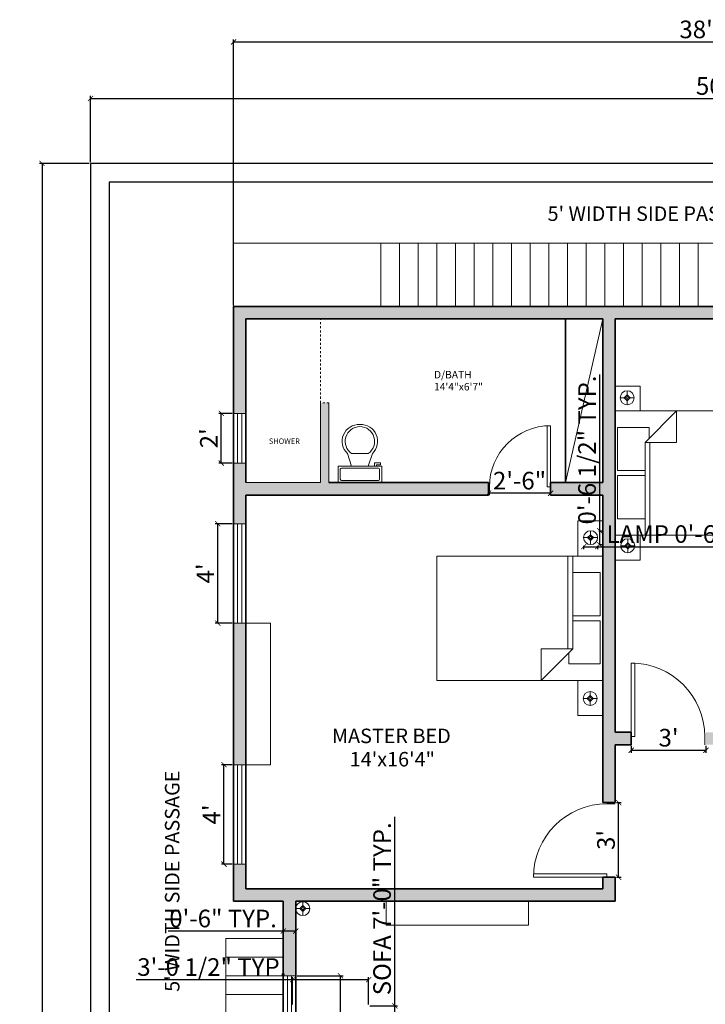
# Model space of a CAD drawing. Units: inches. Extents: x 3799 to 20199, y 1682 to 8087.
# Tile 12 of 30: x 10985 to 11315, y 2798 to 3273. Entities that reach past the tile are written whole.
import ezdxf

# ---------------------------------------------------------------- set-up
doc = ezdxf.new("R2010")
doc.units = ezdxf.units.IN
doc.linetypes.add('JIS_02_1.0', pattern=[2, 1, -1])
for name, color, linetype, lineweight in [('A-ANNO-DIMS', 2, 'Continuous', 18), ('A-ANNO-TEXT', 7, 'Continuous', 18), ('A-AREA-IDEN', 7, 'Continuous', 18), ('A-DOOR', 3, 'Continuous', 18), ('A-FLOR-CASE', 32, 'Continuous', 18), ('A-FLOR-FIXT', 9, 'Continuous', 18), ('A-FLOR-FIXT-HIDN', 9, 'JIS_02_1.0', 13), ('A-FLOR-STRS', 41, 'Continuous', 18), ('A-FURN', 8, 'Continuous', 18), ('A-GLAZ', 152, 'Continuous', 18), ('A-WALL', 7, 'Continuous', 35), ('A-WALL-PATT', 252, 'Continuous', 13), ('C-PROP', 7, 'Continuous', 25)]:
    doc.layers.add(name, color=color, linetype=linetype, lineweight=lineweight)
doc.styles.get("Standard").update_dxf_attribs({"font": 'arial.ttf'})
doc.dimstyles.new('ISO-25', dxfattribs={"dimtxt": 8.5, "dimasz": 2.5, "dimexe": 1.25, "dimexo": 0.625, "dimtad": 1, "dimdec": 0, "dimlunit": 3, "dimtxsty": 'Standard', "dimblk": 'ARCHTICK', "dimcen": 2.5, "dimadec": 0, "dimazin": 0, "dimtfac": 1, "dimtdec": 0, "dimtmove": 0, "dimatfit": 3, "dimfxl": 1, "dimarcsym": 0})

# ---------------------------------------------------------------- blocks, each defined once
blk = doc.blocks.new('*U48')
for p, q in [((-750, 0), (-750, -100)), ((0, 0), (0, -100))]:
    blk.add_line(p, q)
blk.add_lwpolyline([(0, 0), (0, 750), (-43.75, 750), (-43.75, 0)], close=True)
blk.add_arc((0, 0), 750, 90, 180)
blk = doc.blocks.new('*U49')
for p, q in [((0, 0), (0, -100)), ((900, 0), (900, -100))]:
    blk.add_line(p, q)
blk.add_lwpolyline([(0, 0), (0, 900), (43.75, 900), (43.75, 0)], close=True)
blk.add_arc((0, 0), 900, 0, 90)
blk = doc.blocks.new('*U52')
for p, q in [((-900, 0), (-900, 100)), ((0, 0), (0, 100))]:
    blk.add_line(p, q)
blk.add_lwpolyline([(0, 0), (0, -900), (-43.75, -900), (-43.75, 0)], close=True)
blk.add_arc((0, 0), 900, 180, 270)
blk = doc.blocks.new('Bed - Queen')
for p, q in [((0, -80.00003), (0, 0)), ((0, 0), (59.99999, 0)), ((59.99999, 0), (59.99999, -80.00003)), ((7.99999, -1.2), (28.79998, -1.2)), ((7.99999, -14.4), (7.99999, -1.2)), ((28.79998, -1.2), (28.79998, -14.4)), ((31.19999, -1.2), (51.99999, -1.2)), ((31.19999, -14.4), (31.19999, -1.2)), ((51.99999, -1.2), (51.99999, -16.4)), ((0, -14.4), (44.8, -14.4)), ((44.8, -16.8), (0, -16.8)), ((59.99999, -29.6), (44.8, -14.4)), ((44.8, -14.4), (44.8, -29.6)), ((51.99999, -16.4), (46.79936, -16.4)), ((44.8, -29.6), (59.99999, -29.6)), ((59.99999, -80.00003), (0, -80.00003))]:
    blk.add_line(p, q)
blk = doc.blocks.new('*U59')
for p, q in [((9.5, -6), (9.5, -2)), ((-10, -8.5), (-8, -8.5)), ((-10, -9.5), (-10, -8.5)), ((-7, -9.5), (-10, -9.5)), ((-8, -8.5), (-8, -8)), ((-7, -8), (-7, -9.5)), ((-4, -8), (-6, -14)), ((4, -8), (6, -14)), ((4, -14), (-4, -14))]:
    blk.add_line(p, q)
blk.add_lwpolyline([(10.5, -8), (10.5, 0), (-10.5, 0), (-10.5, -8)], close=True)
for points in [[(-9.5, -2), (-9.5, -6)], [(8.5, -1), (-8.5, -1)], [(-8.5, -7), (8.5, -7)]]:
    blk.add_lwpolyline(points)
for centre, radius, start, end in [((-8.625, -1.875), 0.8839, 81.8699, 188.1301), ((8.625, -1.875), 0.8839, 351.8699, 98.1301), ((-8.625, -6.125), 0.8839, 171.869898, 278.1301), ((8.625, -6.125), 0.8839, 261.8699, 8.1301), ((-0.4772, -19.9188), 8.0953, 133.01722, 273.38), ((0.0374, -19.8731), 7.127, 124.50543, 269.7), ((-0.0373, -19.8731), 7.127, 270.3, 55.4946), ((0.4773, -19.9188), 8.0953, 266.62, 46.9828)]:
    blk.add_arc(centre, radius, start, end)
blk = doc.blocks.new('_ArchTick')
at = {"color": 0, "linetype": 'ByBlock', "const_width": 0.15}
blk.add_lwpolyline([(-0.5, -0.5), (0.5, 0.5)], dxfattribs=at)
blk = doc.blocks.new('*D72')
at = {"layer": 'A-ANNO-DIMS', "color": 0, "lineweight": -2, "transparency": 16777216}
for p, q in [((11087.23, 2913.95), (11082, 2913.95)), ((11083.25, 2865.95), (11083.25, 2913.95)), ((11087.23, 2865.95), (11082, 2865.95))]:
    blk.add_line(p, q, dxfattribs=at)
at = {"layer": 'Defpoints', "color": 0, "transparency": 16777216}
for p in [(11083.25, 2913.95), (11087.85, 2913.95), (11087.85, 2865.95)]:
    blk.add_point(p, dxfattribs=at)
at = {"layer": 'A-ANNO-DIMS', "color": 0, "lineweight": -2, "transparency": 16777216, "xscale": 2.5, "yscale": 2.5, "zscale": 2.5}
for p, rotation in [((11083.25, 2913.95), 90), ((11083.25, 2865.95), 270)]:
    blk.add_blockref('_ArchTick', p, dxfattribs=dict(at, rotation=rotation))
at = {"layer": 'A-ANNO-DIMS', "color": 0, "transparency": 16777216, "insert": (11078.37, 2889.95), "char_height": 8.5, "attachment_point": 5, "rotation": 90}
blk.add_mtext("4'", dxfattribs=at)
blk = doc.blocks.new('*D73')
at = {"layer": 'A-ANNO-DIMS', "color": 0, "lineweight": -2, "transparency": 16777216}
for p, q in [((11087.23, 3030.25), (11079, 3030.25)), ((11080.25, 2982.25), (11080.25, 3030.25)), ((11087.23, 2982.25), (11079, 2982.25))]:
    blk.add_line(p, q, dxfattribs=at)
at = {"layer": 'Defpoints', "color": 0, "transparency": 16777216}
for p in [(11080.25, 3030.25), (11087.85, 3030.25), (11087.85, 2982.25)]:
    blk.add_point(p, dxfattribs=at)
at = {"layer": 'A-ANNO-DIMS', "color": 0, "lineweight": -2, "transparency": 16777216, "xscale": 2.5, "yscale": 2.5, "zscale": 2.5}
for p, rotation in [((11080.25, 3030.25), 90), ((11080.25, 2982.25), 270)]:
    blk.add_blockref('_ArchTick', p, dxfattribs=dict(at, rotation=rotation))
at = {"layer": 'A-ANNO-DIMS', "color": 0, "transparency": 16777216, "insert": (11075.37, 3006.25), "char_height": 8.5, "attachment_point": 5, "rotation": 90}
blk.add_mtext("4'", dxfattribs=at)
blk = doc.blocks.new('*D74')
at = {"layer": 'A-ANNO-DIMS', "color": 0, "lineweight": -2, "transparency": 16777216}
for p, q in [((11087.23, 3083.46), (11080.71, 3083.46)), ((11081.96, 3059.46), (11081.96, 3083.46)), ((11087.23, 3059.46), (11080.71, 3059.46))]:
    blk.add_line(p, q, dxfattribs=at)
at = {"layer": 'Defpoints', "color": 0, "transparency": 16777216}
for p in [(11081.96, 3083.46), (11087.85, 3083.46), (11087.85, 3059.46)]:
    blk.add_point(p, dxfattribs=at)
at = {"layer": 'A-ANNO-DIMS', "color": 0, "lineweight": -2, "transparency": 16777216, "xscale": 2.5, "yscale": 2.5, "zscale": 2.5}
for p, rotation in [((11081.96, 3083.46), 90), ((11081.96, 3059.46), 270)]:
    blk.add_blockref('_ArchTick', p, dxfattribs=dict(at, rotation=rotation))
at = {"layer": 'A-ANNO-DIMS', "color": 0, "transparency": 16777216, "insert": (11077.07, 3071.46), "char_height": 8.5, "attachment_point": 5, "rotation": 90}
blk.add_mtext("2'", dxfattribs=at)
blk = doc.blocks.new('*D77')
at = {"layer": 'A-ANNO-DIMS', "color": 0, "lineweight": -2, "transparency": 16777216}
for p, q in [((11018.23, 3204.07), (10994.27, 3204.07)), ((10995.52, 3204.07), (10995.52, 2124.07)), ((11018.23, 2124.07), (10994.27, 2124.07))]:
    blk.add_line(p, q, dxfattribs=at)
at = {"layer": 'Defpoints', "color": 0, "transparency": 16777216}
for p in [(11018.85, 3204.07), (10995.52, 2124.07), (11018.85, 2124.07)]:
    blk.add_point(p, dxfattribs=at)
at = {"layer": 'A-ANNO-DIMS', "color": 0, "lineweight": -2, "transparency": 16777216, "xscale": 2.5, "yscale": 2.5, "zscale": 2.5}
for p, rotation in [((10995.52, 3204.07), 90), ((10995.52, 2124.07), 270)]:
    blk.add_blockref('_ArchTick', p, dxfattribs=dict(at, rotation=rotation))
at = {"layer": 'A-ANNO-DIMS', "color": 0, "transparency": 16777216, "insert": (10990.56, 2664.07), "char_height": 8.5, "attachment_point": 5, "rotation": 90}
blk.add_mtext("90'", dxfattribs=at)
blk = doc.blocks.new('*D78')
at = {"layer": 'A-ANNO-DIMS', "color": 0, "lineweight": -2, "transparency": 16777216}
for p, q in [((11018.85, 3204.7), (11018.85, 3236.64)), ((11618.85, 3204.7), (11618.85, 3236.64)), ((11018.85, 3235.39), (11618.85, 3235.39))]:
    blk.add_line(p, q, dxfattribs=at)
at = {"layer": 'Defpoints', "color": 0, "transparency": 16777216}
for p in [(11618.85, 3235.39), (11018.85, 3204.07), (11618.85, 3204.07)]:
    blk.add_point(p, dxfattribs=at)
at = {"layer": 'A-ANNO-DIMS', "color": 0, "lineweight": -2, "transparency": 16777216, "xscale": 2.5, "yscale": 2.5, "zscale": 2.5, "rotation": 180}
blk.add_blockref('_ArchTick', (11018.85, 3235.39), dxfattribs=at)
at = {"layer": 'A-ANNO-DIMS', "color": 0, "lineweight": -2, "transparency": 16777216, "xscale": 2.5, "yscale": 2.5, "zscale": 2.5}
blk.add_blockref('_ArchTick', (11618.85, 3235.39), dxfattribs=at)
at = {"layer": 'A-ANNO-DIMS', "color": 0, "transparency": 16777216, "insert": (11318.85, 3240.35), "char_height": 8.5, "attachment_point": 5}
blk.add_mtext("50'", dxfattribs=at)
blk = doc.blocks.new('*D85')
at = {"layer": 'A-ANNO-DIMS', "color": 0, "lineweight": -2, "transparency": 16777216}
for p, q in [((11272.48, 2895.64), (11274.76, 2895.64)), ((11273.51, 2859.64), (11273.51, 2895.64)), ((11272.48, 2859.64), (11274.76, 2859.64))]:
    blk.add_line(p, q, dxfattribs=at)
at = {"layer": 'Defpoints', "color": 0, "transparency": 16777216}
for p in [(11271.85, 2895.64), (11273.51, 2895.64), (11271.85, 2859.64)]:
    blk.add_point(p, dxfattribs=at)
at = {"layer": 'A-ANNO-DIMS', "color": 0, "lineweight": -2, "transparency": 16777216, "xscale": 2.5, "yscale": 2.5, "zscale": 2.5}
for p, rotation in [((11273.51, 2895.64), 90), ((11273.51, 2859.64), 270)]:
    blk.add_blockref('_ArchTick', p, dxfattribs=dict(at, rotation=rotation))
at = {"layer": 'A-ANNO-DIMS', "color": 0, "transparency": 16777216, "insert": (11268.54, 2877.64), "char_height": 8.5, "attachment_point": 5, "rotation": 90}
blk.add_mtext("3'", dxfattribs=at)
blk = doc.blocks.new('*D86')
at = {"layer": 'A-ANNO-DIMS', "color": 0, "lineweight": -2, "transparency": 16777216}
for p, q in [((11279.6, 2922.98), (11279.6, 2919.65)), ((11315.6, 2922.98), (11315.6, 2919.65)), ((11279.6, 2920.9), (11315.6, 2920.9))]:
    blk.add_line(p, q, dxfattribs=at)
at = {"layer": 'Defpoints', "color": 0, "transparency": 16777216}
for p in [(11279.6, 2923.61), (11315.6, 2923.61), (11315.6, 2920.9)]:
    blk.add_point(p, dxfattribs=at)
at = {"layer": 'A-ANNO-DIMS', "color": 0, "lineweight": -2, "transparency": 16777216, "xscale": 2.5, "yscale": 2.5, "zscale": 2.5, "rotation": 180}
blk.add_blockref('_ArchTick', (11279.6, 2920.9), dxfattribs=at)
at = {"layer": 'A-ANNO-DIMS', "color": 0, "lineweight": -2, "transparency": 16777216, "xscale": 2.5, "yscale": 2.5, "zscale": 2.5}
blk.add_blockref('_ArchTick', (11315.6, 2920.9), dxfattribs=at)
at = {"layer": 'A-ANNO-DIMS', "color": 0, "transparency": 16777216, "insert": (11297.6, 2925.87), "char_height": 8.5, "attachment_point": 5}
blk.add_mtext("3'", dxfattribs=at)
blk = doc.blocks.new('*D87')
at = {"layer": 'A-ANNO-DIMS', "color": 0, "lineweight": -2, "transparency": 16777216}
for p, q in [((11210.75, 3044.7), (11210.75, 3046.2)), ((11240.75, 3044.7), (11240.75, 3046.2)), ((11240.75, 3044.95), (11210.75, 3044.95))]:
    blk.add_line(p, q, dxfattribs=at)
at = {"layer": 'Defpoints', "color": 0, "transparency": 16777216}
for p in [(11210.75, 3044.95), (11210.75, 3044.07), (11240.75, 3044.07)]:
    blk.add_point(p, dxfattribs=at)
at = {"layer": 'A-ANNO-DIMS', "color": 0, "lineweight": -2, "transparency": 16777216, "xscale": 2.5, "yscale": 2.5, "zscale": 2.5, "rotation": 180}
blk.add_blockref('_ArchTick', (11210.75, 3044.95), dxfattribs=at)
at = {"layer": 'A-ANNO-DIMS', "color": 0, "lineweight": -2, "transparency": 16777216, "xscale": 2.5, "yscale": 2.5, "zscale": 2.5}
blk.add_blockref('_ArchTick', (11240.75, 3044.95), dxfattribs=at)
at = {"layer": 'A-ANNO-DIMS', "color": 0, "transparency": 16777216, "insert": (11225.75, 3049.91), "char_height": 8.5, "attachment_point": 5}
blk.add_mtext('2\'-6"', dxfattribs=at)
blk = doc.blocks.new('Lamp - Table')
for p, q in [((-1, 0), (-7, 0)), ((0, 3), (-3, 0)), ((-3, 0), (0, -3)), ((0, 7), (0, 1)), ((3, 0), (0, 3)), ((0, -3), (3, 0)), ((1, 0), (7, 0)), ((0, -1), (0, -7))]:
    blk.add_line(p, q)
for radius in [7, 1]:
    blk.add_circle((0, 0), radius)
blk = doc.blocks.new('WIN-24IN-6IN-FRAME')
for p, q in [((6, 24), (0, 24)), ((2, 24), (2, 0)), ((4, 24), (4, 0)), ((6, 0), (0, 0))]:
    blk.add_line(p, q)
blk = doc.blocks.new('WIN-48IN-6IN-FRAME')
for p, q in [((0, 0), (0, 6)), ((48, 0), (48, 6)), ((48, 4), (0, 4)), ((48, 2), (0, 2))]:
    blk.add_line(p, q)
blk = doc.blocks.new('WIN-144IN-6IN-FRAME')
for p, q in [((0, 6), (0, 0)), ((144, 6), (144, 0)), ((144, 4), (0, 4)), ((144, 2), (0, 2))]:
    blk.add_line(p, q)
blk = doc.blocks.new('*D246')
at = {"layer": 'A-ANNO-DIMS', "color": 0, "lineweight": -2, "transparency": 16777216}
for p, q in [((11256.67, 3019.5), (11256.67, 3017.87)), ((11256.67, 3019.12), (11263.41, 3019.12)), ((11263.41, 3019.5), (11263.41, 3017.87)), ((11263.41, 3019.12), (11374.03, 3019.12))]:
    blk.add_line(p, q, dxfattribs=at)
at = {"layer": 'Defpoints', "color": 0, "transparency": 16777216}
for p in [(11256.67, 3020.13), (11263.41, 3020.13), (11263.41, 3019.12)]:
    blk.add_point(p, dxfattribs=at)
at = {"layer": 'A-ANNO-DIMS', "color": 0, "lineweight": -2, "transparency": 16777216, "xscale": 2.5, "yscale": 2.5, "zscale": 2.5, "rotation": 180}
blk.add_blockref('_ArchTick', (11256.67, 3019.12), dxfattribs=at)
at = {"layer": 'A-ANNO-DIMS', "color": 0, "lineweight": -2, "transparency": 16777216, "xscale": 2.5, "yscale": 2.5, "zscale": 2.5}
blk.add_blockref('_ArchTick', (11263.41, 3019.12), dxfattribs=at)
at = {"layer": 'A-ANNO-DIMS', "color": 0, "transparency": 16777216, "insert": (11319.97, 3024.14), "char_height": 8.5, "attachment_point": 5}
blk.add_mtext('LAMP 0\'-6 1/2" TYP.', dxfattribs=at)
blk = doc.blocks.new('*D247')
at = {"layer": 'A-ANNO-DIMS', "color": 0, "lineweight": -2, "transparency": 16777216}
for p, q in [((11264.42, 3026.87), (11264.42, 3102.23)), ((11264.03, 3026.87), (11265.67, 3026.87)), ((11264.42, 3020.13), (11264.42, 3026.87)), ((11264.03, 3020.13), (11265.67, 3020.13))]:
    blk.add_line(p, q, dxfattribs=at)
at = {"layer": 'Defpoints', "color": 0, "transparency": 16777216}
for p in [(11263.41, 3026.87), (11264.42, 3026.87), (11263.41, 3020.13)]:
    blk.add_point(p, dxfattribs=at)
at = {"layer": 'A-ANNO-DIMS', "color": 0, "lineweight": -2, "transparency": 16777216, "xscale": 2.5, "yscale": 2.5, "zscale": 2.5}
for p, rotation in [((11264.42, 3026.87), 90), ((11264.42, 3020.13), 270)]:
    blk.add_blockref('_ArchTick', p, dxfattribs=dict(at, rotation=rotation))
at = {"layer": 'A-ANNO-DIMS', "color": 0, "transparency": 16777216, "insert": (11259.4, 3065.8), "char_height": 8.5, "attachment_point": 5, "rotation": 90}
blk.add_mtext('0\'-6 1/2" TYP.', dxfattribs=at)
blk = doc.blocks.new('*D258')
at = {"layer": 'A-ANNO-DIMS', "color": 0, "lineweight": -2, "transparency": 16777216}
for p, q in [((11165.6, 2797.6), (11165.6, 2888.75)), ((11153.62, 2797.6), (11166.85, 2797.6)), ((11165.6, 2713.6), (11165.6, 2797.6)), ((11153.62, 2713.6), (11166.85, 2713.6))]:
    blk.add_line(p, q, dxfattribs=at)
at = {"layer": 'Defpoints', "color": 0, "transparency": 16777216}
for p in [(11153, 2797.6), (11165.6, 2797.6), (11153, 2713.6)]:
    blk.add_point(p, dxfattribs=at)
at = {"layer": 'A-ANNO-DIMS', "color": 0, "lineweight": -2, "transparency": 16777216, "xscale": 2.5, "yscale": 2.5, "zscale": 2.5}
for p, rotation in [((11165.6, 2797.6), 90), ((11165.6, 2713.6), 270)]:
    blk.add_blockref('_ArchTick', p, dxfattribs=dict(at, rotation=rotation))
at = {"layer": 'A-ANNO-DIMS', "color": 0, "transparency": 16777216, "insert": (11160.58, 2844.42), "char_height": 8.5, "attachment_point": 5, "rotation": 90}
blk.add_mtext('SOFA 7\'-0" TYP.', dxfattribs=at)
blk = doc.blocks.new('*D259')
at = {"layer": 'A-ANNO-DIMS', "color": 0, "lineweight": -2, "transparency": 16777216}
for p, q in [((11116.33, 2810.2), (11040.97, 2810.2)), ((11116.33, 2798.22), (11116.33, 2811.45)), ((11153, 2810.2), (11116.33, 2810.2)), ((11153, 2798.22), (11153, 2811.45))]:
    blk.add_line(p, q, dxfattribs=at)
at = {"layer": 'Defpoints', "color": 0, "transparency": 16777216}
for p in [(11116.33, 2810.2), (11116.33, 2797.6), (11153, 2797.6)]:
    blk.add_point(p, dxfattribs=at)
at = {"layer": 'A-ANNO-DIMS', "color": 0, "lineweight": -2, "transparency": 16777216, "xscale": 2.5, "yscale": 2.5, "zscale": 2.5, "rotation": 180}
blk.add_blockref('_ArchTick', (11116.33, 2810.2), dxfattribs=at)
at = {"layer": 'A-ANNO-DIMS', "color": 0, "lineweight": -2, "transparency": 16777216, "xscale": 2.5, "yscale": 2.5, "zscale": 2.5}
blk.add_blockref('_ArchTick', (11153, 2810.2), dxfattribs=at)
at = {"layer": 'A-ANNO-DIMS', "color": 0, "transparency": 16777216, "insert": (11077.4, 2815.22), "char_height": 8.5, "attachment_point": 5}
blk.add_mtext('3\'-0 1/2" TYP.', dxfattribs=at)
blk = doc.blocks.new('*D354')
at = {"layer": 'A-ANNO-DIMS', "color": 0, "lineweight": -2, "transparency": 16777216}
for p, q in [((11118.48, 2812.07), (11140.7, 2812.07)), ((11139.45, 2668.07), (11139.45, 2812.07)), ((11118.48, 2668.07), (11140.7, 2668.07))]:
    blk.add_line(p, q, dxfattribs=at)
at = {"layer": 'Defpoints', "color": 0, "transparency": 16777216}
for p in [(11117.85, 2812.07), (11139.45, 2812.07), (11117.85, 2668.07)]:
    blk.add_point(p, dxfattribs=at)
at = {"layer": 'A-ANNO-DIMS', "color": 0, "lineweight": -2, "transparency": 16777216, "xscale": 2.5, "yscale": 2.5, "zscale": 2.5}
for p, rotation in [((11139.45, 2812.07), 90), ((11139.45, 2668.07), 270)]:
    blk.add_blockref('_ArchTick', p, dxfattribs=dict(at, rotation=rotation))
at = {"layer": 'A-ANNO-DIMS', "color": 0, "transparency": 16777216, "insert": (11134.43, 2740.07), "char_height": 8.5, "attachment_point": 5, "rotation": 90}
blk.add_mtext('WINDOW 12\'-0" TYP.', dxfattribs=at)
blk = doc.blocks.new('*D355')
at = {"layer": 'A-ANNO-DIMS', "color": 0, "lineweight": -2, "transparency": 16777216}
for p, q in [((11111.85, 2833.67), (11056.29, 2833.67)), ((11111.85, 2812.7), (11111.85, 2834.92)), ((11117.85, 2833.67), (11111.85, 2833.67)), ((11117.85, 2812.7), (11117.85, 2834.92))]:
    blk.add_line(p, q, dxfattribs=at)
at = {"layer": 'Defpoints', "color": 0, "transparency": 16777216}
for p in [(11111.85, 2833.67), (11111.85, 2812.07), (11117.85, 2812.07)]:
    blk.add_point(p, dxfattribs=at)
at = {"layer": 'A-ANNO-DIMS', "color": 0, "lineweight": -2, "transparency": 16777216, "xscale": 2.5, "yscale": 2.5, "zscale": 2.5, "rotation": 180}
blk.add_blockref('_ArchTick', (11111.85, 2833.67), dxfattribs=at)
at = {"layer": 'A-ANNO-DIMS', "color": 0, "lineweight": -2, "transparency": 16777216, "xscale": 2.5, "yscale": 2.5, "zscale": 2.5}
blk.add_blockref('_ArchTick', (11117.85, 2833.67), dxfattribs=at)
at = {"layer": 'A-ANNO-DIMS', "color": 0, "transparency": 16777216, "insert": (11082.82, 2838.64), "char_height": 8.5, "attachment_point": 5}
blk.add_mtext('0\'-6" TYP.', dxfattribs=at)
blk = doc.blocks.new('*D373')
at = {"layer": 'A-ANNO-DIMS', "color": 0, "lineweight": -2, "transparency": 16777216}
for p, q in [((11087.85, 3135.7), (11087.85, 3263.92)), ((11549.85, 3135.7), (11549.85, 3263.92)), ((11087.85, 3262.67), (11549.85, 3262.67))]:
    blk.add_line(p, q, dxfattribs=at)
at = {"layer": 'Defpoints', "color": 0, "transparency": 16777216}
for p in [(11549.85, 3262.67), (11087.85, 3135.07), (11549.85, 3135.07)]:
    blk.add_point(p, dxfattribs=at)
at = {"layer": 'A-ANNO-DIMS', "color": 0, "lineweight": -2, "transparency": 16777216, "xscale": 2.5, "yscale": 2.5, "zscale": 2.5, "rotation": 180}
blk.add_blockref('_ArchTick', (11087.85, 3262.67), dxfattribs=at)
at = {"layer": 'A-ANNO-DIMS', "color": 0, "lineweight": -2, "transparency": 16777216, "xscale": 2.5, "yscale": 2.5, "zscale": 2.5}
blk.add_blockref('_ArchTick', (11549.85, 3262.67), dxfattribs=at)
at = {"layer": 'A-ANNO-DIMS', "color": 0, "transparency": 16777216, "insert": (11318.85, 3267.64), "char_height": 8.5, "attachment_point": 5}
blk.add_mtext('38\'-6"', dxfattribs=at)

msp = doc.modelspace()

# ---------------------------------------------------------------- hatches: boundary and pattern name
at = {"layer": 'A-WALL-PATT'}
h = msp.add_hatch(color=256, dxfattribs=at)
h.dxf.hatch_style = 1
h.paths.add_polyline_path([(11549.85, 2537.07), (11543.85, 2537.07), (11543.85, 2493.07), (11500.92, 2493.07), (11500.92, 2487.07), (11543.85, 2487.07), (11543.85, 2331.07), (11512.59, 2331.07), (11512.59, 2325.07), (11549.85, 2325.07)])
h.paths.add_polyline_path([(11404.92, 2493.07), (11369.85, 2493.07), (11369.85, 2535.29), (11363.85, 2535.29), (11363.85, 2493.07), (11359.67, 2493.07), (11359.67, 2487.07), (11404.92, 2487.07)])
h.paths.add_polyline_path([(11347.67, 2493.07), (11315.85, 2493.07), (11315.85, 2481.32), (11321.85, 2481.32), (11321.85, 2487.07), (11347.67, 2487.07)])
h.paths.add_polyline_path([(11246.96, 2394.07), (11231.85, 2394.07), (11231.85, 2493.07), (11126.81, 2493.07), (11126.81, 2487.07), (11225.85, 2487.07), (11225.85, 2325.07), (11315.85, 2325.07), (11315.85, 2331.07), (11231.85, 2331.07), (11231.85, 2388.07), (11246.96, 2388.07)])
h.paths.add_polyline_path([(11368.59, 2331.07), (11321.85, 2331.07), (11321.85, 2421.32), (11319.79, 2421.32), (11315.85, 2421.32), (11315.85, 2394.07), (11306.96, 2394.07), (11306.96, 2392.01), (11306.96, 2388.07), (11315.85, 2388.07), (11315.85, 2325.07), (11368.59, 2325.07)])
h.paths.add_polyline_path([(11211.5, 2599.62), (11175.25, 2599.62), (11175.25, 2594.62), (11206.5, 2594.62), (11206.5, 2541.62), (11137.5, 2541.62), (11137.5, 2594.62), (11145.25, 2594.62), (11145.25, 2599.62), (11132.5, 2599.62), (11132.5, 2536.62), (11211.5, 2536.62)], flags=17)
h.paths.add_polyline_path([(11278.96, 2650.07), (11117.85, 2650.07), (11117.85, 2668.07), (11111.85, 2668.07), (11111.85, 2650.07), (11087.85, 2650.07), (11087.85, 2526.57), (11093.85, 2526.57), (11093.85, 2644.07), (11278.96, 2644.07)])
h.paths.add_polyline_path([(11096.81, 2491.01), (11096.81, 2493.07), (11093.85, 2493.07), (11093.85, 2496.57), (11087.85, 2496.57), (11087.85, 2487.07), (11096.81, 2487.07)])
h.paths.add_polyline_path([(11445.85, 3087.71), (11439.85, 3087.71), (11439.85, 2949.07), (11343.85, 2949.07), (11343.85, 2929.61), (11315.6, 2929.61), (11315.6, 2923.61), (11343.85, 2923.61), (11343.85, 2840.12), (11349.85, 2840.12), (11349.85, 2943.07), (11507.11, 2943.07), (11507.11, 2949.07), (11445.85, 2949.07), (11445.85, 3015.07), (11543.85, 3015.07), (11543.85, 2992.92), (11549.85, 2992.92), (11549.85, 3108.28), (11543.85, 3108.28), (11543.85, 3021.07), (11515.89, 3021.07), (11515.89, 3049.36), (11511.89, 3049.36), (11511.89, 3021.07), (11445.85, 3021.07)])
h.paths.add_polyline_path([(11549.85, 3135.07), (11408.12, 3135.07), (11408.12, 3129.07), (11439.85, 3129.07), (11439.85, 3117.71), (11443.79, 3117.71), (11445.85, 3117.71), (11445.85, 3129.07), (11504.47, 3129.07), (11504.47, 3099.65), (11508.47, 3099.65), (11508.47, 3129.07), (11543.85, 3129.07), (11543.85, 3126.28), (11549.85, 3126.28)])
h.paths.add_polyline_path([(11324.12, 3135.07), (11087.85, 3135.07), (11087.85, 3083.46), (11093.85, 3083.46), (11093.85, 3129.07), (11265.85, 3129.07), (11265.85, 3050.07), (11240.75, 3050.07), (11240.75, 3044.07), (11265.85, 3044.07), (11265.85, 2895.64), (11271.85, 2895.64), (11271.85, 2923.61), (11279.6, 2923.61), (11279.6, 2929.61), (11271.85, 2929.61), (11271.85, 3129.07), (11324.12, 3129.07)])
h.paths.add_polyline_path([(11210.75, 3050.07), (11133.85, 3050.07), (11133.85, 3088.63), (11129.85, 3088.54), (11129.85, 3050.07), (11093.85, 3050.07), (11093.85, 3059.46), (11087.85, 3059.46), (11087.85, 3030.25), (11093.85, 3030.25), (11093.85, 3044.07), (11210.75, 3044.07)], flags=17)
h.paths.add_polyline_path([(11093.85, 2982.25), (11087.85, 2982.25), (11087.85, 2913.95), (11093.85, 2913.95)], flags=17)
h.paths.add_polyline_path([(11271.85, 2859.64), (11265.85, 2859.64), (11265.85, 2854.07), (11093.85, 2854.07), (11093.85, 2865.95), (11087.85, 2865.95), (11087.85, 2848.07), (11111.85, 2848.07), (11111.85, 2812.07), (11117.85, 2812.07), (11117.85, 2848.07), (11271.85, 2848.07)])
h.paths.add_polyline_path([(11549.85, 2847.23), (11543.85, 2847.23), (11543.85, 2799.07), (11349.85, 2799.07), (11349.85, 2804.12), (11343.85, 2804.12), (11343.85, 2753.07), (11349.85, 2753.07), (11349.85, 2793.07), (11543.85, 2793.07), (11543.85, 2752.31), (11549.85, 2752.31)])
h.paths.add_polyline_path([(11549.85, 2692.31), (11543.85, 2692.31), (11543.85, 2650.07), (11343.85, 2650.07), (11338.96, 2650.07), (11338.96, 2644.07), (11349.85, 2644.07), (11363.85, 2644.07), (11363.85, 2608.29), (11369.85, 2608.29), (11369.85, 2644.07), (11543.85, 2644.07), (11543.85, 2621.07), (11549.85, 2621.07)])

# ---------------------------------------------------------------- linework, layer by layer
at = {"layer": 'A-FLOR-CASE'}
for p, q in [((11093.85, 2982.25), (11105.71, 2982.25)), ((11105.71, 2982.25), (11105.71, 2913.95)), ((11105.71, 2913.95), (11093.85, 2913.95)), ((11161.39, 2848.07), (11161.39, 2836.54)), ((11230.09, 2836.54), (11230.09, 2848.07)), ((11161.39, 2836.54), (11230.09, 2836.54))]:
    msp.add_line(p, q, dxfattribs=at)
at = {"layer": 'A-FLOR-FIXT'}
for p, q in [((11265.85, 3129.07), (11247.85, 3050.07)), ((11129.85, 3088.54), (11129.85, 3050.07)), ((11133.85, 3088.63), (11133.85, 3050.07)), ((11129.85, 3050.07), (11093.85, 3050.07))]:
    msp.add_line(p, q, dxfattribs=at)
at = {"layer": 'A-FLOR-FIXT-HIDN'}
for p, q in [((11129.85, 3088.54), (11129.85, 3129.07)), ((11133.85, 3088.63), (11129.85, 3088.54))]:
    msp.add_line(p, q, dxfattribs=at)
at = {"layer": 'A-FLOR-STRS'}
for p, q in [((11087.85, 3135.07), (11087.85, 3165.66)), ((11087.85, 3165.66), (11442.62, 3165.66)), ((11158.86, 3165.66), (11158.86, 3135.07)), ((11167.86, 3165.66), (11167.86, 3135.07)), ((11176.86, 3165.66), (11176.86, 3135.07)), ((11185.86, 3165.66), (11185.86, 3135.07)), ((11194.86, 3165.66), (11194.86, 3135.07)), ((11203.86, 3165.66), (11203.86, 3135.07)), ((11212.86, 3165.66), (11212.86, 3135.07)), ((11221.86, 3165.66), (11221.86, 3135.07)), ((11230.86, 3165.66), (11230.86, 3135.07)), ((11239.86, 3165.66), (11239.86, 3135.07)), ((11248.86, 3165.66), (11248.86, 3135.07)), ((11257.86, 3165.66), (11257.86, 3135.07)), ((11266.86, 3165.66), (11266.86, 3135.07)), ((11275.86, 3165.66), (11275.86, 3135.07)), ((11284.86, 3165.66), (11284.86, 3135.07)), ((11293.86, 3165.66), (11293.86, 3135.07)), ((11302.86, 3165.66), (11302.86, 3135.07)), ((11311.86, 3165.66), (11311.86, 3135.07)), ((11111.85, 2830.07), (11084.17, 2830.07)), ((11084.17, 2650.07), (11084.17, 2830.07)), ((11111.85, 2821.07), (11084.17, 2821.07)), ((11111.85, 2812.07), (11084.17, 2812.07)), ((11111.85, 2803.07), (11084.17, 2803.07))]:
    msp.add_line(p, q, dxfattribs=at)
at = {"layer": 'A-FURN'}
for points in [[(11271.85, 3084.65), (11283.85, 3084.65), (11283.85, 3096.65), (11271.85, 3096.65)], [(11265.85, 3014.64), (11253.85, 3014.64), (11253.85, 3031.64), (11265.85, 3031.64)], [(11271.85, 3024.65), (11283.85, 3024.65), (11283.85, 3012.65), (11271.85, 3012.65)], [(11265.85, 2954.64), (11253.85, 2954.64), (11253.85, 2937.64), (11265.85, 2937.64)]]:
    msp.add_lwpolyline(points, close=True, dxfattribs=at)
at = {"layer": 'A-WALL'}
for p, q in [((11549.85, 3135.07), (11087.85, 3135.07)), ((11087.85, 3135.07), (11087.85, 2848.07)), ((11093.85, 3129.07), (11093.85, 3050.07)), ((11265.85, 3129.07), (11093.85, 3129.07)), ((11247.85, 3129.07), (11247.85, 3050.07)), ((11265.85, 3129.07), (11265.85, 3050.07)), ((11271.85, 3129.07), (11271.85, 2929.61)), ((11439.85, 3129.07), (11271.85, 3129.07)), ((11210.75, 3050.07), (11133.85, 3050.07)), ((11210.75, 3050.07), (11210.75, 3044.07)), ((11265.85, 3050.07), (11240.75, 3050.07)), ((11240.75, 3050.07), (11240.75, 3044.07)), ((11093.85, 3044.07), (11093.85, 2854.07)), ((11210.75, 3044.07), (11093.85, 3044.07)), ((11265.85, 3044.07), (11240.75, 3044.07)), ((11265.85, 3044.07), (11265.85, 2895.64)), ((11279.6, 2929.61), (11271.85, 2929.61)), ((11279.6, 2929.61), (11279.6, 2923.61)), ((11271.85, 2923.61), (11271.85, 2895.64)), ((11279.6, 2923.61), (11271.85, 2923.61)), ((11265.85, 2895.64), (11271.85, 2895.64)), ((11265.85, 2859.64), (11271.85, 2859.64)), ((11265.85, 2859.64), (11265.85, 2854.07)), ((11271.85, 2859.64), (11271.85, 2848.07)), ((11265.85, 2854.07), (11093.85, 2854.07)), ((11111.85, 2848.07), (11087.85, 2848.07)), ((11111.85, 2848.07), (11111.85, 2650.07)), ((11271.85, 2848.07), (11117.85, 2848.07)), ((11117.85, 2848.07), (11117.85, 2650.07))]:
    msp.add_line(p, q, dxfattribs=at)
at = {"layer": 'C-PROP'}
for p, q in [((11618.85, 3204.07), (11018.85, 3204.07)), ((11018.85, 3204.07), (11018.85, 2124.07)), ((11609.85, 3195.07), (11027.85, 3195.07)), ((11027.85, 3195.07), (11027.85, 2133.07))]:
    msp.add_line(p, q, dxfattribs=at)

# ---------------------------------------------------------------- block references
at = {"layer": 'A-DOOR', "xscale": 0.0393700787401575, "yscale": 0.0393700787401575, "zscale": 0.0393700787401575}
for name, p in [('*U48', (11240.75, 3048.01)), ('*U49', (11279.6, 2927.54))]:
    msp.add_blockref(name, p, dxfattribs=at)
at = {"layer": 'A-DOOR', "xscale": 0.0393700787401575, "yscale": 0.0393700787401575, "zscale": 0.0393700787401575, "rotation": 270}
msp.add_blockref('*U52', (11267.92, 2859.64), dxfattribs=at)
at = {"layer": 'A-FLOR-FIXT', "rotation": 180}
msp.add_blockref('*U59', (11148.78, 3050.07), dxfattribs=at)
at = {"layer": 'A-FURN', "xscale": 0.4812244018485111, "yscale": 0.4812244018485111, "zscale": 0.4812244018485111}
for p in [(11277.65, 3091.01), (11260.04, 3023.5), (11277.91, 3019.61), (11259.82, 2945.91), (11121.22, 2844.49)]:
    msp.add_blockref('Lamp - Table', p, dxfattribs=at)
at = {"layer": 'A-FURN'}
for p, rotation in [((11271.85, 3024.65), 90), ((11265.85, 3014.64), 270)]:
    msp.add_blockref('Bed - Queen', p, dxfattribs=dict(at, rotation=rotation))
at = {"layer": 'A-GLAZ'}
msp.add_blockref('WIN-24IN-6IN-FRAME', (11087.85, 3059.46), dxfattribs=at)
at = {"layer": 'A-GLAZ', "rotation": 90}
for name, p in [('WIN-48IN-6IN-FRAME', (11093.85, 2982.25)), ('WIN-48IN-6IN-FRAME', (11093.85, 2865.94)), ('WIN-144IN-6IN-FRAME', (11117.85, 2668.07))]:
    msp.add_blockref(name, p, dxfattribs=at)

# ---------------------------------------------------------------- texts
at = {"layer": 'A-ANNO-TEXT'}
for rotation, p in [(0.0019, (11239.28, 3176.34)), (90.0019, (11061.79, 2804.36))]:
    msp.add_text("5' WIDTH SIDE PASSAGE", height=7, rotation=rotation, dxfattribs=at).set_placement(p)
at = {"layer": 'A-AREA-IDEN'}
for s, height, rotation, p in [('D/BATH', 3.621, 0.0167, (11184.52, 3100.33)), ('14\'4"x6\'7"', 3.621, 0.0167, (11184.52, 3094.52)), ('SHOWER', 2.63, 0.0019, (11104.89, 3068.74)), ('MASTER BED', 7, 0.0019, (11135.33, 2924.35)), ('    14\'x16\'4"', 7, 0.0019, (11135.33, 2913.1))]:
    msp.add_text(s, height=height, rotation=rotation, dxfattribs=at).set_placement(p)

# ---------------------------------------------------------------- dimensions: what is measured, and where the dimension line sits
at = {"layer": 'A-ANNO-DIMS'}
for base, p1, p2, override, picture, middle in [((11549.85, 3262.67), (11087.85, 3135.07), (11549.85, 3135.07), {"dimdec": 1, "dimlfac": 1, "dimrnd": 0, "dimzin": 1, "dimdsep": 46, "dimlunit": 4, "dimfrac": 2}, '*D373', (11318.85, 3267.64)), ((11618.85, 3235.39), (11018.85, 3204.07), (11618.85, 3204.07), {"dimclrd": 0, "dimclre": 0, "dimclrt": 0}, '*D78', (11318.85, 3240.35)), ((11210.75, 3044.95), (11240.75, 3044.07), (11210.75, 3044.07), {"dimclrd": 0, "dimclre": 0, "dimclrt": 0}, '*D87', (11225.75, 3049.91)), ((11315.6, 2920.9), (11279.6, 2923.61), (11315.6, 2923.61), {"dimclrd": 0, "dimclre": 0, "dimclrt": 0}, '*D86', (11297.6, 2925.87))]:
    dim = msp.add_linear_dim(base=base, p1=p1, p2=p2, dimstyle='ISO-25', override=override, dxfattribs=at)
    dim.commit()
    dim.dimension.update_dxf_attribs({"geometry": picture, "text_midpoint": middle})
for base, p1, p2, picture, middle in [((10995.52, 2124.07), (11018.85, 3204.07), (11018.85, 2124.07), '*D77', (10990.56, 2664.07)), ((11081.96, 3083.46), (11087.85, 3059.46), (11087.85, 3083.46), '*D74', (11077.07, 3071.46)), ((11080.25, 3030.25), (11087.85, 2982.25), (11087.85, 3030.25), '*D73', (11075.37, 3006.25)), ((11083.25, 2913.95), (11087.85, 2865.95), (11087.85, 2913.95), '*D72', (11078.37, 2889.95)), ((11273.51, 2895.64), (11271.85, 2859.64), (11271.85, 2895.64), '*D85', (11268.54, 2877.64))]:
    dim = msp.add_linear_dim(base=base, p1=p1, p2=p2, angle=90, dimstyle='ISO-25', override={"dimclrd": 0, "dimclre": 0, "dimclrt": 0}, dxfattribs=at)
    dim.commit()
    dim.dimension.update_dxf_attribs({"geometry": picture, "text_midpoint": middle})
for base, p1, p2, angle, text, picture, middle in [((11264.42, 3026.87), (11263.41, 3020.13), (11263.41, 3026.87), 90, '<> TYP.', '*D247', (11259.4, 3065.8)), ((11165.6, 2797.6), (11153, 2713.6), (11153, 2797.6), 90, 'SOFA <> TYP.', '*D258', (11160.58, 2844.42)), ((11111.85, 2833.67), (11117.85, 2812.07), (11111.85, 2812.07), 180, '<> TYP.', '*D355', (11082.82, 2838.64)), ((11116.33, 2810.2), (11153, 2797.6), (11116.33, 2797.6), 180, '<> TYP.', '*D259', (11077.4, 2815.22)), ((11139.45, 2812.07), (11117.85, 2668.07), (11117.85, 2812.07), 90, 'WINDOW <> TYP.', '*D354', (11134.43, 2740.07))]:
    dim = msp.add_linear_dim(base=base, p1=p1, p2=p2, angle=angle, text=text, dimstyle='ISO-25', override={"dimdec": 1, "dimlfac": 1, "dimrnd": 0, "dimzin": 1, "dimdsep": 46, "dimlunit": 4, "dimfrac": 2}, dxfattribs=at)
    dim.commit()
    dim.dimension.update_dxf_attribs({"geometry": picture, "text_midpoint": middle})
dim = msp.add_linear_dim(base=(11263.41, 3019.12), p1=(11256.67, 3020.13), p2=(11263.41, 3020.13), text='LAMP <> TYP.', dimstyle='ISO-25', override={"dimdec": 1, "dimlfac": 1, "dimrnd": 0, "dimzin": 1, "dimdsep": 46, "dimlunit": 4, "dimfrac": 2}, dxfattribs=at)
dim.commit()
dim.dimension.update_dxf_attribs({"geometry": '*D246', "text_midpoint": (11319.97, 3024.14)})

doc.saveas('drawing.dxf')
